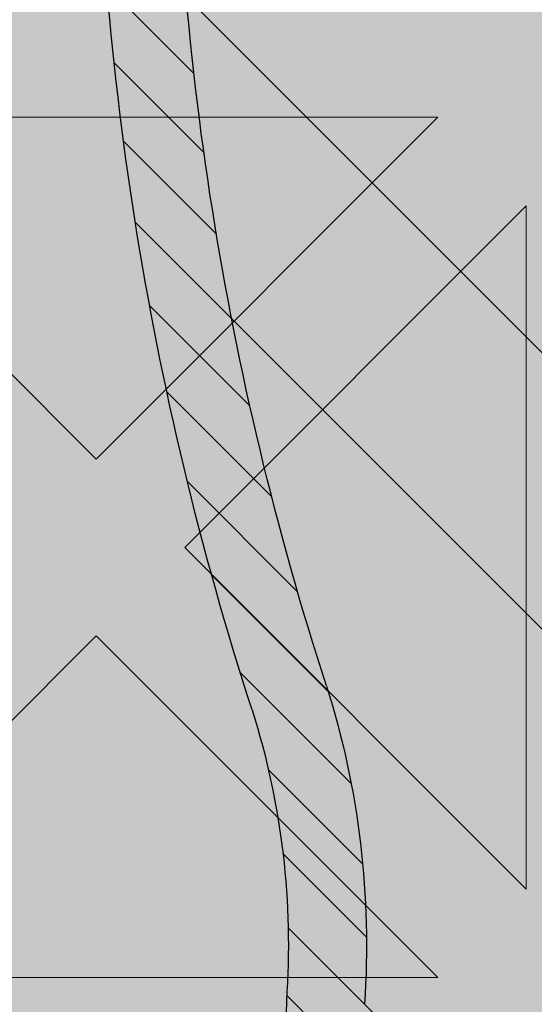
# Model space of a CAD drawing. Units: inches. Extents: x 844 to 2234, y 346 to 1084.
# Tile 70 of 93: x 2000.116 to 2001.166, y 694.327 to 696.335. Entities that reach past the tile are written whole.
import ezdxf

# ---------------------------------------------------------------- set-up
doc = ezdxf.new("R2010")
doc.units = ezdxf.units.IN
doc.header["$MEASUREMENT"] = 0
for name, color, linetype, lineweight in [('A-ANNO-DIMS', 2, 'Continuous', 18), ('furniture', 8, 'Continuous', 18), ('RA-AP-01$0$INT', 35, 'Continuous', 5)]:
    doc.layers.add(name, color=color, linetype=linetype, lineweight=lineweight)
doc.layers.add('RA-AP-01$0$FURN', color=3, linetype='Continuous')
doc.layers.add('RA-AP-01$0$WOOD', color=64, linetype='Continuous')
doc.styles.get("Standard").update_dxf_attribs({"font": 'arial.ttf'})
doc.dimstyles.get("Standard").update_dxf_attribs({"dimtxt": 6, "dimasz": 3, "dimexe": 0.18, "dimexo": 0.0625, "dimgap": 0.09, "dimtad": 0, "dimtih": 1, "dimtoh": 1, "dimdec": 1, "dimzin": 0, "dimdsep": 46, "dimlunit": 3, "dimtxsty": 'Standard', "dimblk": 'ARCHTICK', "dimcen": 0.09, "dimadec": 0, "dimazin": 0, "dimtfac": 1, "dimtdec": 1, "dimtofl": 0, "dimtmove": 0, "dimatfit": 3, "dimfxl": 1, "dimtolj": 1, "dimtzin": 0, "dimarcsym": 0})

# ---------------------------------------------------------------- blocks, each defined once
blk = doc.blocks.new('A$C18D01794')
at = {"layer": 'RA-AP-01$0$INT'}
h = blk.add_hatch(color=256, dxfattribs=at)
h.paths.add_polyline_path([(4.585917135068448, -6.356712009588273), (4.614201406330596, -6.356712009589021), (4.668846067270487, -6.411356670531338), (4.723490728212344, -6.356712009591912), (4.771774999457151, -6.35671200959319), (4.826419660396886, -6.411356670535356), (4.862780050090322, -6.374996280843536), (4.844495778842715, -6.356712009595112), (4.862780050090411, -6.356712009595595), (4.905206456960182, -6.399138416468211), (4.947632863832445, -6.356712009597838), (4.965917135079675, -6.356712009598322), (4.947632863831759, -6.374996280845421), (4.983993253523576, -6.411356670538857), (5.038637914464627, -6.356712009600247), (5.08692218571208, -6.356712009601523), (5.141566846649976, -6.411356670541852), (5.196211507589851, -6.356712009604411), (5.224495778822615, -6.356712009605161), (4.905206456953975, -6.676001331473793)])
h.paths.add_polyline_path([(4.895206456956031, -6.637717060225675), (4.895206456958921, -6.528427738347902), (4.840561796018589, -6.583072399285802)], flags=16)
h.paths.add_polyline_path([(4.915206456955638, -6.637717060226121), (4.969851117895509, -6.583072399288678), (4.915206456957609, -6.528427738348344)], flags=16)
h.paths.add_polyline_path([(4.826419660395175, -6.568930263661755), (4.881064321335613, -6.514285602723745), (4.771774999456703, -6.514285602720857)], flags=16)
h.paths.add_polyline_path([(4.983993253519558, -6.568930263665262), (5.038637914460456, -6.514285602726792), (4.929348592581548, -6.514285602724816)], flags=16)
h.paths.add_polyline_path([(4.881064321336025, -6.494285602723742), (4.826419660397532, -6.439640941782821), (4.771774999457062, -6.494285602720859)], flags=16)
h.paths.add_polyline_path([(4.929348592582019, -6.494285602724817), (5.038637914460982, -6.494285602726792), (4.983993253522945, -6.439640941786327)], flags=16)
h.paths.add_polyline_path([(4.895206456960191, -6.480143467100443), (4.895206456962115, -6.407422687715913), (4.876922185715016, -6.389138416467584), (4.840561796021581, -6.425498806159401)], flags=16)
h.paths.add_polyline_path([(4.915206456958487, -6.480143467100889), (4.969851117899527, -6.425498806162279), (4.933490728206909, -6.389138416468043), (4.9152064569598, -6.40742268771434)], flags=16)
h.paths.add_polyline_path([(4.757632863832376, -6.480143467096812), (4.812277524772842, -6.425498806158772), (4.757632863834348, -6.370854145217844)], flags=16)
h.paths.add_polyline_path([(4.737632863832376, -6.480143467096286), (4.737632863834348, -6.370854145217375), (4.682988202893906, -6.425498806155385)], flags=16)
h.paths.add_polyline_path([(5.05278005008503, -6.480143467103376), (5.052780050087917, -6.370854145224413), (4.998135389146995, -6.425498806162908)], flags=16)
h.paths.add_polyline_path([(5.072780050085024, -6.480143467103744), (5.127424711025931, -6.42549880616527), (5.072780050087916, -6.370854145224832)], flags=16)
h.paths.add_polyline_path([(4.935917135072783, -6.706712009592292), (5.255206456948811, -6.387422687716309), (5.255206456948932, -6.415706958964177), (5.200561796010279, -6.470351619902839), (5.255206456949403, -6.524996280841948), (5.25520645694961, -6.5732805520894), (5.200561796009787, -6.627925213029239), (5.236922185702417, -6.664285602721864), (5.255206456949919, -6.646001331474357), (5.255206456949998, -6.664285602721898), (5.212780050078687, -6.706712009592262), (5.25520645695036, -6.749138416463932), (5.255206456950438, -6.767422687711313), (5.236922185702424, -6.749138416463297), (5.200561796009796, -6.785498806155928), (5.255206456950753, -6.840143467096874), (5.25520645695096, -6.888427738341682), (5.200561796010322, -6.943072399282328), (5.255206456951428, -6.997717060223427), (5.255206456951547, -7.026001331471006)])
h.paths.add_polyline_path([(5.042988202883395, -6.785498806155427), (5.097632863823085, -6.840143467095101), (5.097632863822622, -6.730854145216193)], flags=16)
h.paths.add_polyline_path([(5.028846067259663, -6.771356670531693), (5.083490728198774, -6.716712009592573), (4.974201406321001, -6.716712009593042)], flags=16)
h.paths.add_polyline_path([(5.117632863823087, -6.840143467095186), (5.172277524762331, -6.785498806155926), (5.11763286382262, -6.730854145216225)], flags=16)
h.paths.add_polyline_path([(5.08349072819877, -6.696712009593886), (5.028846067259652, -6.642067348654775), (4.974201406320998, -6.696712009593438)], flags=16)
h.paths.add_polyline_path([(5.131774999446817, -6.854285602718917), (5.186419660386065, -6.799640941779662), (5.241064321325782, -6.854285602719365)], flags=17)
h.paths.add_polyline_path([(5.131774999446228, -6.716712009592374), (5.186419660386065, -6.771356670532194), (5.222780050079488, -6.734996280838764), (5.204495778832781, -6.716712009592063)], flags=16)
h.paths.add_polyline_path([(5.097632863822613, -6.682569873970264), (5.097632863823061, -6.573280552091354), (5.042988202883383, -6.627925213031044)], flags=16)
h.paths.add_polyline_path([(5.131774999446899, -6.874285602718915), (5.241064321325809, -6.874285602719364), (5.186419660386591, -6.928930263658598)], flags=17)
h.paths.add_polyline_path([(5.131774999446226, -6.696712009594078), (5.204495778830767, -6.696712009594374), (5.22278005007868, -6.67842773834687), (5.186419660386049, -6.642067348654249)], flags=16)
h.paths.add_polyline_path([(5.11763286382262, -6.682569873970225), (5.17227752476232, -6.627925213030515), (5.117632863823064, -6.573280552091267)], flags=16)
h.paths.add_polyline_path([(5.186419660386069, -6.613783077405491), (5.241064321325754, -6.559138416465795), (5.131774999446791, -6.559138416466263)], flags=16)
h.paths.add_polyline_path([(5.131774999446872, -6.539138416466263), (5.24106432132578, -6.539138416465794), (5.186419660386554, -6.484493755526573)], flags=16)
h.paths.add_polyline_path([(5.255206456951811, -7.08742268770861), (5.255206456951895, -7.106712009588038), (4.555206456956052, -7.106712009588038), (4.555206456956136, -7.087422687708617), (4.905206456953973, -6.737422687710788)])
h.paths.add_polyline_path([(4.983993253513404, -6.8444937555241), (4.92934859257295, -6.899138416462108), (5.03863791445186, -6.899138416465014)], flags=16)
h.paths.add_polyline_path([(4.969851117889988, -6.83035161990006), (4.915206456952556, -6.775706958960171), (4.915206456949648, -6.884996280837944)], flags=16)
h.paths.add_polyline_path([(4.929348592572535, -6.919138416462105), (4.983993253511019, -6.973783077403037), (5.038637914451496, -6.919138416465012)], flags=16)
h.paths.add_polyline_path([(5.052780050074912, -6.93328055208906), (4.998135389134438, -6.987925213027088), (5.052780050072919, -7.042569873968025)], flags=16)
h.paths.add_polyline_path([(5.07278005007491, -6.933280552089588), (5.072780050072918, -7.042569873968497), (5.127424711013374, -6.987925213030498)], flags=16)
h.paths.add_polyline_path([(4.89520645695295, -6.775706958959721), (4.840561796013067, -6.830351619897157), (4.895206456950961, -6.884996280837494)], flags=16)
h.paths.add_polyline_path([(4.915206456948365, -6.933280552085403), (4.915206456946434, -7.006001331471951), (4.933490728192729, -7.024285602719066), (4.969851117886972, -6.987925213026453)], flags=16)
h.paths.add_polyline_path([(4.881064321327021, -6.899138416461022), (4.82641966038902, -6.84449375552057), (4.771774999448108, -6.899138416459029)], flags=16)
h.paths.add_polyline_path([(4.895206456950073, -6.933280552084951), (4.840561796009022, -6.987925213023558), (4.876922185700835, -7.024285602716997), (4.895206456948749, -7.006001331469487)], flags=16)
h.paths.add_polyline_path([(4.983993253510392, -7.0020673486505), (4.947632863816944, -7.038427738342319), (4.965917135064043, -7.05671200959023), (5.038637914448995, -7.056712009591555)], flags=16)
h.paths.add_polyline_path([(4.881064321326543, -6.91913841646102), (4.771774999447578, -6.919138416459031), (4.826419660385607, -6.973783077399508)], flags=16)
h.paths.add_polyline_path([(4.905206456946447, -7.014285602717636), (4.862780050074785, -7.056712009588352), (4.947632863816685, -7.056712009589775)], flags=16)
h.paths.add_polyline_path([(5.14156684663679, -7.002067348654549), (5.086922185696452, -7.056712009592438), (5.196211507574223, -7.056712009594425)], flags=16)
h.paths.add_polyline_path([(4.8264196603837, -7.002067348646972), (4.771774999442643, -7.056712009585575), (4.8444957788276, -7.056712009587508), (4.862780050075511, -7.038427738340416)], flags=16)
h.paths.add_polyline_path([(4.812277524760289, -6.98792521302292), (4.757632863822258, -6.933280552082447), (4.757632863819352, -7.042569873961408)], flags=16)
h.paths.add_polyline_path([(4.73763286382226, -6.933280552082079), (4.682988202881349, -6.987925213020536), (4.737632863819352, -7.04256987396099)], flags=16)
h.paths.add_polyline_path([(4.723490728195188, -7.056712009584289), (4.668846067257299, -7.002067348643949), (4.614201406317417, -7.056712009581383)], flags=16)
h.paths.add_polyline_path([(4.597632863829262, -6.706712009592262), (4.555206456957951, -6.664285602721896), (4.555206456958029, -6.646001331474357), (4.573490728205535, -6.664285602721864), (4.609851117898167, -6.627925213029238), (4.555206456958338, -6.573280552089402), (4.555206456958546, -6.524996280841952), (4.60985111789767, -6.470351619902839), (4.555206456959015, -6.415706958964177), (4.555206456959138, -6.387422687716309), (4.874495778835167, -6.70671200959229), (4.5552064569564, -7.026001331471015), (4.555206456956523, -6.997717060223433), (4.609851117897629, -6.94307239928233), (4.555206456956988, -6.888427738341681), (4.555206456957198, -6.840143467096881), (4.609851117898153, -6.78549880615593), (4.573490728205528, -6.749138416463297), (4.555206456957507, -6.76742268771132), (4.555206456957585, -6.749138416463933)])
h.paths.add_polyline_path([(4.712780050085332, -6.730854145216195), (4.712780050084863, -6.840143467095105), (4.767424711024555, -6.785498806155427)], flags=16)
h.paths.add_polyline_path([(4.726922185709173, -6.716712009592573), (4.781566846648288, -6.771356670531693), (4.836211507586949, -6.716712009593043)], flags=16)
h.paths.add_polyline_path([(4.692780050085327, -6.730854145216225), (4.638135389145619, -6.785498806155928), (4.692780050084865, -6.840143467095185)], flags=16)
h.paths.add_polyline_path([(4.726922185709182, -6.696712009593886), (4.836211507586949, -6.696712009593436), (4.7815668466483, -6.642067348654773)], flags=16)
h.paths.add_polyline_path([(4.678637914461726, -6.71671200959237), (4.605917135075169, -6.716712009592063), (4.587632863828464, -6.734996280838766), (4.623993253521887, -6.771356670532195)], flags=16)
h.paths.add_polyline_path([(4.712780050085336, -6.68256987397026), (4.767424711024568, -6.627925213031042), (4.71278005008489, -6.573280552091352)], flags=16)
h.paths.add_polyline_path([(4.678637914461726, -6.696712009594076), (4.623993253521899, -6.642067348654247), (4.587632863829271, -6.67842773834687), (4.605917135077185, -6.696712009594376)], flags=16)
h.paths.add_polyline_path([(4.692780050085336, -6.682569873970228), (4.692780050084889, -6.573280552091267), (4.638135389145632, -6.627925213030515)], flags=16)
h.paths.add_polyline_path([(4.623993253521885, -6.799640941779662), (4.678637914461131, -6.854285602718915), (4.56934859258217, -6.854285602719365)], flags=17)
h.paths.add_polyline_path([(4.623993253521901, -6.613783077405509), (4.678637914461158, -6.559138416466263), (4.569348592582195, -6.559138416465795)], flags=16)
h.paths.add_polyline_path([(4.678637914461051, -6.874285602718915), (4.623993253521361, -6.928930263658598), (4.569348592582143, -6.874285602719364)], flags=17)
h.paths.add_polyline_path([(4.678637914461076, -6.539138416466263), (4.623993253521399, -6.484493755526573), (4.569348592582167, -6.539138416465796)], flags=16)
h = blk.add_hatch(color=256, dxfattribs=at)
h.paths.add_polyline_path([(5.028846067259997, -6.642067348655121), (4.974201406321342, -6.696712009593783), (5.083490728199115, -6.69671200959423)])
h.paths.add_polyline_path([(4.974201406321344, -6.716712009593388), (5.028846067260004, -6.771356670532039), (5.083490728199117, -6.716712009592919)])
h.paths.add_polyline_path([(5.042988202883738, -6.785498806155768), (5.097632863823428, -6.840143467095449), (5.097632863822963, -6.73085414521654)])
h.paths.add_polyline_path([(5.117632863822961, -6.730854145216568), (5.117632863823428, -6.840143467095531), (5.172277524762674, -6.785498806156272)])
h.paths.add_polyline_path([(5.131774999446572, -6.716712009592718), (5.186419660386406, -6.77135667053254), (5.222780050079831, -6.734996280839116), (5.204495778833122, -6.716712009592409)])
h.paths.add_polyline_path([(5.236922185702764, -6.749138416463644), (5.200561796010139, -6.785498806156274), (5.255206456949971, -6.840143467096101), (5.255206456950271, -6.76742268771115)])
h.paths.add_polyline_path([(5.186419660386412, -6.799640941780006), (5.131774999447164, -6.854285602719262), (5.241064321326123, -6.854285602719711)])
h.paths.add_polyline_path([(5.131774999447238, -6.874285602719261), (5.186419660386934, -6.928930263658944), (5.241064321326153, -6.874285602719709)])
h.paths.add_polyline_path([(5.200561796010663, -6.943072399282675), (5.255206456949324, -6.997717060221329), (5.255206456949777, -6.888427738343558)])
h.paths.add_polyline_path([(5.21278005007903, -6.706712009592607), (5.255206456950223, -6.749138416463798), (5.255206456950696, -6.664285602721891)])
h.paths.add_polyline_path([(5.13177499944657, -6.696712009594424), (5.204495778831106, -6.696712009594723), (5.222780050079024, -6.678427738347219), (5.186419660386397, -6.642067348654592)])
h.paths.add_polyline_path([(5.117632863823405, -6.573280552091611), (5.117632863822955, -6.682569873970578), (5.172277524762665, -6.627925213030859)])
h.paths.add_polyline_path([(5.042988202883727, -6.627925213031387), (5.097632863822957, -6.682569873970603), (5.097632863823407, -6.573280552091697)])
h.paths.add_polyline_path([(5.131774999447135, -6.559138416466609), (5.186419660386394, -6.613783077405857), (5.241064321326097, -6.559138416466144)])
h.paths.add_polyline_path([(5.200561796010128, -6.627925213029584), (5.236922185702758, -6.664285602722211), (5.255206456950264, -6.646001331474705), (5.255206456949948, -6.573280552089752)])
h.paths.add_polyline_path([(5.186419660386895, -6.484493755526919), (5.131774999447213, -6.539138416466609), (5.241064321326127, -6.539138416466142)])
h.paths.add_polyline_path([(5.200561796010624, -6.470351619903183), (5.255206456949745, -6.524996280842298), (5.255206456949276, -6.415706958964523)])
for p, q in [((5.131774999446792, -6.559138416466263), (5.241064321325755, -6.559138416465795)), ((5.131774999446792, -6.559138416466263), (5.186419660386049, -6.613783077405509)), ((5.241064321325755, -6.559138416465795), (5.186419660386049, -6.613783077405509)), ((5.117632863823062, -6.573280552091267), (5.172277524762319, -6.627925213030515)), ((5.117632863823062, -6.573280552091267), (5.117632863822614, -6.68256987397023)), ((5.117632863822614, -6.68256987397023), (5.172277524762319, -6.627925213030515)), ((5.131774999446228, -6.696712009594078), (5.186419660386053, -6.642067348654247)), ((5.186419660386051, -6.642067348654247), (5.222780050078681, -6.67842773834687)), ((5.204495778831179, -6.696712009594376), (5.131774999446228, -6.696712009594078))]:
    blk.add_line(p, q, dxfattribs=at)
blk = doc.blocks.new('A$C32926AE1')
at = {"layer": 'RA-AP-01$0$WOOD'}
h = blk.add_hatch(color=256, dxfattribs=at)
h.dxf.hatch_style = 1
h.paths.add_polyline_path([(5.157430609644524, 4.573483066760929, -0.1009492694046607), (5.155401577623758, 4.593365984175333, -0.1842662638101597), (5.172249623284174, 4.638795604568598, 0.2056608120311276), (5.179560981299304, 4.661316324430096, 0.3614336704623542), (5.134352340494423, 4.706524965234944, 0.2056608120311297), (5.111831620632933, 4.699213607219793, -0.1842662638101113), (5.066402000239693, 4.682365561559342, -0.1055311479399994), (5.045656153913092, 4.68467289944697, 0.1567636581983829), (4.763886414745334, 4.684672899446966, -0.1055311479399895), (4.743140568418733, 4.68236556155934, -0.1842662638100833), (4.6977109480255, 4.69921360721979, 0.2056608120302612), (4.675190228164109, 4.706524965234949, 0.3614336704708441), (4.629981587358889, 4.66131632442871, 0.2056608120245944), (4.637292945374126, 4.638795604567974, -0.1842662638101024), (4.654140991034615, 4.59336598417475, -0.1009492694055169), (4.652111959013835, 4.573483066760181, 0.021410119221476), (4.629748025606143, 4.156712009541676, 0.0214101192214795), (4.652111959013809, 3.739940952323101, -0.1009492694059586), (4.654140991034615, 3.720058034908448, -0.1842662638100975), (4.637292945374126, 3.674628414515226, 0.2056608120245705), (4.629981587358889, 3.652107694654492, 0.3614336704708879), (4.675190228164113, 3.606899053848249, 0.2056608120302384), (4.697710948025501, 3.614210411863408, -0.1842662638100995), (4.743140568418738, 3.63105845752386, -0.1055311479402541), (4.763886414745388, 3.628751119636215, 0.1567636581983776), (5.045656153913137, 3.628751119636244, -0.1055311479397538), (5.066402000239692, 3.631058457523857, -0.1842662638101067), (5.111831620632931, 3.614210411863407, 0.2056608120310924), (5.134352340494417, 3.606899053848256, 0.3614336704624001), (5.179560981299307, 3.652107694653103, 0.2056608120311314), (5.172249623284175, 3.6746284145146, -0.1842662638101402), (5.155401577623758, 3.72005803490786, -0.1009492694051366), (5.15743060964455, 3.739940952322354, 0.0214101192215073), (5.179794543052287, 4.156712009541468, 0.0214101192215252)])
h.paths.add_polyline_path([(4.639748609479751, 4.156712009541513, 0.0213537860821624), (4.661970494867118, 3.741887061152232, -0.094075836301374), (4.664143710413708, 3.7196126951003, -0.1824818158568985), (4.644813765429836, 3.668037719127816, 0.2056608120245319), (4.639939526753007, 3.653023905887301, 0.3614336704710246), (4.676106439397173, 3.616856993242342, 0.2056608120302234), (4.691120252638095, 3.621731231919122, -0.1824818158602558), (4.742695228611606, 3.641061176902986, -0.1029891339458722), (4.766991894714349, 3.638256818950944, 0.156709409989566), (5.042550673941472, 3.638256818950105, -0.102989133958497), (5.066847340047078, 3.641061176902949, -0.1824818158594995), (5.118422316020358, 3.621731231919103, 0.2056608120311416), (5.133436129261316, 3.616856993242346, 0.3614336704621468), (5.169603041905217, 3.653023905886178, 0.2056608120310986), (5.164728803228477, 3.668037719127177, -0.1824818158565612), (5.145398858244737, 3.719612695099578, -0.0940758363009313), (5.147572073791232, 3.741887061151398, 0.0213537860822023), (5.169793959178681, 4.156712009541451, 0.0213537860822226), (5.147572073791203, 4.571536957931898, -0.0940758363005034), (5.145398858244737, 4.59381132398362, -0.1824818158565587), (5.164728803228476, 4.645386299956021, 0.2056608120311045), (5.169603041905216, 4.66040011319702, 0.3614336704621845), (5.133436129261313, 4.696567025840856, 0.2056608120310773), (5.118422316020359, 4.691692787164098, -0.182481815859508), (5.066847340047078, 4.67236284218025, -0.1029891339584606), (5.04255067394148, 4.675167200133092, 0.156709409989566), (4.766991894714357, 4.675167200132257, -0.1029891339458842), (4.742695228611611, 4.672362842180213, -0.1824818158602725), (4.691120252638095, 4.691692787164077, 0.2056608120302152), (4.676106439397174, 4.696567025840858, 0.3614336704710363), (4.639939526753005, 4.660400113195899, 0.2056608120245495), (4.644813765429837, 4.645386299955384, -0.1824818158568934), (4.664143710413708, 4.593811323982902, -0.0940758363009187), (4.661970494867149, 4.571536957931074, 0.021353786082177)], flags=16)
h.paths.add_polyline_path([(5.129794543052235, 4.432167055276933, -0.0141661062790638), (5.130152669293814, 4.156927903047693, -0.0141661062790647), (5.129794543052234, 3.881688750818433, -0.0785247771143638), (5.10979738006795, 3.755143611847103, 0.0945969212073497), (5.105408519571111, 3.717898134952927, 0.1043170707844957), (5.116074640131521, 3.670385395016088, 0.1043170707864965), (5.068561900193738, 3.681051515576561, 0.09459692119553), (5.031316423304057, 3.676662655080835, -0.1580239521427272), (4.778226145355827, 3.676662655080367, 0.0945969211986668), (4.740980668464973, 3.681051515576592, 0.1043170707882822), (4.693467928526415, 3.670385395015844, 0.1043170707867916), (4.704134049087309, 3.717898134953662, 0.0945969211972894), (4.69974518859162, 3.755143611844042, -0.0785247771163196), (4.679748025606343, 3.881688750818406, -0.0141661062790663), (4.679389899364763, 4.156927903047693, -0.0141661062790672), (4.679748025606343, 4.432167055276998, -0.0785247771163064), (4.699745188591625, 4.55871219425134, 0.094596921197333), (4.704134049087308, 4.595957671141738, 0.1043170707867205), (4.693467928526416, 4.643470411079523, 0.1043170707882628), (4.740980668464965, 4.632804290518776, 0.0945969211988114), (4.778226145355874, 4.637193151015016, -0.158023952142669), (5.031316423304015, 4.637193151014546, 0.0945969211956361), (5.068561900193736, 4.632804290518806, 0.1043170707864979), (5.11607464013152, 4.643470411079278, 0.1043170707844617), (5.105408519571112, 4.595957671142455, 0.0945969212074597), (5.109797380067959, 4.558712194248236, -0.0785247771143467)], flags=0)
h.paths.add_polyline_path([(5.119794532311105, 4.432259799204851, -0.0142000800617244), (5.120156169157484, 4.156927903047701, -0.0142000800617277), (5.119794532311105, 3.881596006890482, -0.0784894509520253), (5.100273383573699, 3.758192358677797, 0.0940138827242913), (5.095413455884425, 3.717477693979438, 0.0606271852308753), (5.099615656341024, 3.686844378806616, 0.0606271852322524), (5.068982341167493, 3.691046579263239, 0.0940138827010453), (5.028267676478798, 3.686186651576848, -0.1580706864508061), (4.781274892180912, 3.686186651576435, 0.0940138827026903), (4.740560227491556, 3.691046579263279, 0.0606271852339895), (4.709926912317155, 3.686844378806508, 0.0606271852329405), (4.714129112773991, 3.717477693980356, 0.094013882701304), (4.709269185087677, 3.758192358669163, -0.0784894509577193), (4.689748036347473, 3.881596006890469, -0.014200080061729), (4.689386399501094, 4.156927903047709, -0.0142000800617217), (4.689748036347473, 4.432259799204808, -0.078489450957724), (4.709269185087651, 4.555663447426125, 0.0940138827014585), (4.714129112773992, 4.596378112114996, 0.0606271852329731), (4.709926912317154, 4.62701142728886, 0.0606271852340196), (4.74056022749157, 4.622809226832087, 0.0940138827024997), (4.781274892180847, 4.627669154518912, -0.1580706864508359), (5.028267676478777, 4.627669154518526, 0.0940138827010946), (5.068982341167492, 4.622809226832129, 0.060627185232254), (5.099615656341024, 4.627011427288751, 0.0606271852308727), (5.095413455884425, 4.59637811211593, 0.0940138827241088), (5.100273383573675, 4.555663447417647, -0.0784894509520978)], flags=0)
h.paths.add_polyline_path([(5.06978912287499, 4.430218106756144, -0.014241683694547), (5.070173729147532, 4.156927903047672, -0.0142416836945458), (5.06978912287499, 3.883637699339223, -0.0800609523125196), (5.052662118612511, 3.773463122773442, 0.0526421978001116), (5.04590916754064, 3.740550867606997, 0.0526421977992423), (5.012996912374707, 3.73379791653534, -0.1583028414718258), (4.796545656286308, 3.73379791653451, 0.0526421978034211), (4.763633401117837, 3.740550867607021, 0.0526421978018622), (4.756880450045755, 3.773463122774558, -0.0800609523117106), (4.739753445783639, 3.883637699339268, -0.0142416836945435), (4.739368839511098, 4.156927903047671, -0.0142416836945477), (4.739753445783639, 4.430218106756155, -0.0800609523116345), (4.75688045004574, 4.540392683320762, 0.052642197801941), (4.763633401117837, 4.573304938488346, 0.0526421978035071), (4.796545656286361, 4.580057889560873, -0.1583028414717561), (5.012996912374669, 4.580057889560039, 0.0526421977993048), (5.04590916754064, 4.57330493848837, 0.0526421978002057), (5.052662118612529, 4.540392683321868, -0.080060952312477)], flags=0)
h.paths.add_polyline_path([(5.049789715110557, 4.43038092723357, -0.0143097550741839), (5.05018085590259, 4.156927903047715, -0.0143097550741854), (5.049789715110558, 3.883474878861827, -0.0800685599149176), (5.03362098255317, 3.779581877367999, 0.0306258898956367), (5.028241146483733, 3.758218888663947, 0.0306258898977031), (5.006878157778253, 3.75283905259408, -0.1583983521624096), (4.802664410878162, 3.752839052594731, 0.0306258898946014), (4.781301422174808, 3.758218888663924, 0.0306258898967912), (4.775921586105202, 3.779581877368794, -0.080068559914251), (4.759752853548071, 3.883474878861786, -0.0143097550741854), (4.759361712756037, 4.156927903047671, -0.0143097550741854), (4.759752853548071, 4.430380927233557, -0.0800685599142479), (4.775921586105193, 4.534273928726546, 0.0306258898968306), (4.781301422174808, 4.555636917431444, 0.0306258898945754), (4.802664410878143, 4.561016753500631, -0.1583983521624168), (5.006878157778244, 4.561016753501291, 0.0306258898977177), (5.028241146483733, 4.555636917431421, 0.0306258898958182), (5.03362098255321, 4.534273928727244, -0.080068559914796)], flags=0)
h.paths.add_polyline_path([(4.999766070382627, 4.428171244713864, -0.0143443147609634), (5.000198441819402, 4.156927903047689, -0.0143443147609612), (4.999766070382627, 3.885684561381556, -0.0784641635803329), (4.987356730658798, 3.799103304488872, -0.1506053783831347), (4.822185837999821, 3.79910330448882, -0.0784641635803318), (4.809776498276007, 3.885684561381509, -0.014344314760963), (4.809344126839227, 4.156927903047677, -0.0143443147609645), (4.809776498276007, 4.428171244713873, -0.0784641635803192), (4.822185837999822, 4.514752501606549, -0.1506053783831338), (4.987356730658798, 4.514752501606494, -0.078464163580285)], flags=0)
h.paths.add_polyline_path([(4.979755254238824, 4.42764379880488, -0.0143772539198268), (4.980205517789977, 4.156927903047693, -0.0143772539198275), (4.979755254238824, 3.886212007290489, -0.0689242507424422), (4.971183264704897, 3.815276770442801, -0.1296645318904179), (4.838359303953726, 3.815276770442746, -0.0689242507424186), (4.829787314419809, 3.886212007290419, -0.0143772539198292), (4.829337050868653, 4.156927903047653, -0.0143772539198325), (4.829787314419809, 4.427643798804946, -0.0689242507424211), (4.838359303953725, 4.498579035652621, -0.1296645318904187), (4.971183264704897, 4.498579035652565, -0.0689242507424401)], flags=0)
h = blk.add_hatch(color=256, dxfattribs=at)
h.dxf.hatch_style = 1
h.paths.add_polyline_path([(5.145398858244737, 4.59381132398362, -0.1824818158565616), (5.164728803228476, 4.645386299956021, 0.2056608120311045), (5.169603041905216, 4.66040011319702, 0.3614336704621845), (5.133436129261313, 4.696567025840856, 0.2056608120310773), (5.118422316020359, 4.691692787164098, -0.182481815859508), (5.066847340047078, 4.67236284218025, -0.1029891339584606), (5.04255067394148, 4.675167200133092, 0.156709409989566), (4.766991894714357, 4.675167200132257, -0.1029891339458842), (4.742695228611611, 4.672362842180213, -0.1824818158602725), (4.691120252638095, 4.691692787164077, 0.2056608120302152), (4.676106439397174, 4.696567025840858, 0.3614336704710363), (4.639939526753005, 4.660400113195899, 0.2056608120245495), (4.644813765429837, 4.645386299955384, -0.1824818158568934), (4.664143710413708, 4.593811323982902, -0.0940758363009187), (4.661970494867149, 4.571536957931074, 0.0213537860821772), (4.639748609479751, 4.156712009541507, 0.0213537860821625), (4.661970494867119, 3.741887061152226, -0.0940758363013071), (4.664143710413708, 3.719612695100309, -0.1824818158569294), (4.644813765429836, 3.668037719127816, 0.2056608120245319), (4.639939526753007, 3.653023905887301, 0.3614336704710246), (4.676106439397173, 3.616856993242342, 0.2056608120302234), (4.691120252638095, 3.621731231919122, -0.1824818158602558), (4.742695228611606, 3.641061176902986, -0.1029891339458722), (4.766991894714349, 3.638256818950944, 0.156709409989566), (5.042550673941472, 3.638256818950105, -0.102989133958497), (5.066847340047078, 3.641061176902949, -0.1824818158594995), (5.118422316020358, 3.621731231919103, 0.2056608120311416), (5.133436129261316, 3.616856993242346, 0.3614336704621468), (5.169603041905217, 3.653023905886178, 0.2056608120310986), (5.164728803228477, 3.668037719127177, -0.1824818158565612), (5.145398858244737, 3.719612695099578, -0.0940758363009313), (5.147572073791232, 3.741887061151398, 0.0213537860822023), (5.169793959178681, 4.156712009541451, 0.0213537860822226), (5.147572073791203, 4.571536957931898, -0.0940758363004996)])
h.paths.add_polyline_path([(5.109797380067958, 4.55871219424824, -0.0785247771143472), (5.129794543052234, 4.432167055276936, -0.0141661062790644), (5.130152669293814, 4.156927903047685, -0.014166106279066), (5.129794543052234, 3.881688750818401, -0.0785247771143517), (5.109797380067946, 3.755143611847092, 0.0945969212073132), (5.105408519571111, 3.717898134952929, 0.1043170707844995), (5.116074640131521, 3.670385395016088, 0.1043170707864965), (5.068561900193738, 3.681051515576561, 0.09459692119553), (5.031316423304057, 3.676662655080835, -0.1580239521427272), (4.778226145355827, 3.676662655080367, 0.0945969211986668), (4.740980668464973, 3.681051515576592, 0.1043170707882822), (4.693467928526415, 3.670385395015844, 0.1043170707867916), (4.704134049087309, 3.717898134953662, 0.0945969211972894), (4.69974518859162, 3.755143611844042, -0.0785247771163196), (4.679748025606343, 3.881688750818406, -0.0141661062790663), (4.679389899364763, 4.156927903047693, -0.0141661062790672), (4.679748025606343, 4.432167055276998, -0.0785247771163064), (4.699745188591625, 4.55871219425134, 0.094596921197333), (4.704134049087308, 4.595957671141738, 0.1043170707867205), (4.693467928526416, 4.643470411079523, 0.1043170707882628), (4.740980668464965, 4.632804290518776, 0.0945969211988114), (4.778226145355874, 4.637193151015016, -0.158023952142669), (5.031316423304015, 4.637193151014546, 0.0945969211956361), (5.068561900193736, 4.632804290518806, 0.1043170707864979), (5.11607464013152, 4.643470411079278, 0.1043170707844617), (5.105408519571112, 4.595957671142455, 0.0945969212074504)], flags=16)
h.paths.add_polyline_path([(5.100273383573655, 4.55566344741771, -0.0784894509521388), (5.119794532311105, 4.432259799204852, -0.0142000800617252), (5.120156169157484, 4.156927903047686, -0.014200080061726), (5.119794532311105, 3.881596006890502, -0.0784894509520446), (5.100273383573696, 3.758192358677786, 0.0940138827242721), (5.095413455884425, 3.717477693979436, 0.0606271852308692), (5.099615656341024, 3.686844378806616, 0.0606271852322522), (5.068982341167493, 3.691046579263239, 0.0940138827010453), (5.028267676478798, 3.686186651576848, -0.1580706864508061), (4.781274892180912, 3.686186651576435, 0.0940138827026903), (4.740560227491556, 3.691046579263279, 0.0606271852339895), (4.709926912317155, 3.686844378806508, 0.0606271852329405), (4.714129112773991, 3.717477693980356, 0.094013882701304), (4.709269185087677, 3.758192358669163, -0.0784894509577193), (4.689748036347473, 3.881596006890469, -0.014200080061729), (4.689386399501094, 4.156927903047709, -0.0142000800617217), (4.689748036347473, 4.432259799204808, -0.078489450957724), (4.709269185087651, 4.555663447426125, 0.0940138827014585), (4.714129112773992, 4.596378112114996, 0.0606271852329731), (4.709926912317154, 4.62701142728886, 0.0606271852340196), (4.74056022749157, 4.622809226832087, 0.0940138827024997), (4.781274892180847, 4.627669154518912, -0.1580706864508359), (5.028267676478777, 4.627669154518526, 0.0940138827010946), (5.068982341167492, 4.622809226832129, 0.060627185232254), (5.099615656341024, 4.627011427288751, 0.0606271852308727), (5.095413455884425, 4.59637811211593, 0.094013882723957)], flags=0)
h.paths.add_polyline_path([(5.04590916754064, 4.57330493848837, 0.0526421978002057), (5.052662118612529, 4.540392683321868, -0.0800609523124783), (5.06978912287499, 4.430218106756142, -0.0142416836945469), (5.070173729147532, 4.156927903047672, -0.0142416836945458), (5.06978912287499, 3.883637699339223, -0.0800609523125196), (5.052662118612511, 3.773463122773442, 0.0526421978001116), (5.04590916754064, 3.740550867606997, 0.0526421977992423), (5.012996912374707, 3.73379791653534, -0.1583028414718258), (4.796545656286308, 3.73379791653451, 0.0526421978034211), (4.763633401117837, 3.740550867607021, 0.0526421978018622), (4.756880450045755, 3.773463122774558, -0.0800609523117106), (4.739753445783639, 3.883637699339268, -0.0142416836945435), (4.739368839511098, 4.156927903047671, -0.0142416836945477), (4.739753445783639, 4.430218106756155, -0.0800609523116345), (4.75688045004574, 4.540392683320762, 0.052642197801941), (4.763633401117837, 4.573304938488346, 0.0526421978035071), (4.796545656286361, 4.580057889560873, -0.1583028414717561), (5.012996912374669, 4.580057889560039, 0.0526421977993048)], flags=0)
h.paths.add_polyline_path([(5.028241146483733, 4.555636917431422, 0.0306258898956949), (5.033620982553182, 4.534273928727329, -0.0800685599148649), (5.049789715110557, 4.430380927233569, -0.0143097550741839), (5.05018085590259, 4.156927903047715, -0.0143097550741854), (5.049789715110558, 3.883474878861827, -0.0800685599149176), (5.03362098255317, 3.779581877367999, 0.0306258898956367), (5.028241146483733, 3.758218888663947, 0.0306258898977031), (5.006878157778253, 3.75283905259408, -0.1583983521624096), (4.802664410878162, 3.752839052594731, 0.0306258898946014), (4.781301422174808, 3.758218888663924, 0.0306258898967912), (4.775921586105202, 3.779581877368794, -0.080068559914251), (4.759752853548071, 3.883474878861786, -0.0143097550741854), (4.759361712756037, 4.156927903047671, -0.0143097550741854), (4.759752853548071, 4.430380927233557, -0.0800685599142479), (4.775921586105193, 4.534273928726546, 0.0306258898968306), (4.781301422174808, 4.555636917431444, 0.0306258898945754), (4.802664410878143, 4.561016753500631, -0.1583983521624168), (5.006878157778244, 4.561016753501291, 0.0306258898977174)], flags=0)
h.paths.add_polyline_path([(4.987356730658798, 4.514752501606494, -0.0784641635803018), (4.999766070382627, 4.428171244713845, -0.0143443147609637), (5.000198441819402, 4.156927903047665, -0.0143443147609622), (4.999766070382628, 3.885684561381514, -0.0784641635802952), (4.987356730658797, 3.799103304488872, -0.1506053783831338), (4.822185837999821, 3.799103304488819, -0.0784641635803342), (4.809776498276007, 3.885684561381512, -0.0143443147609628), (4.809344126839227, 4.156927903047676, -0.0143443147609646), (4.809776498276007, 4.428171244713873, -0.0784641635803192), (4.822185837999822, 4.514752501606549, -0.1506053783831338)], flags=0)
h.paths.add_polyline_path([(4.971183264704897, 4.498579035652566, -0.0689242507424384), (4.979755254238824, 4.427643798804883, -0.0143772539198276), (4.980205517789977, 4.15692790304768, -0.0143772539198258), (4.979755254238823, 3.88621200729051, -0.0689242507424628), (4.971183264704897, 3.815276770442801, -0.129664531890417), (4.838359303953726, 3.815276770442746, -0.0689242507424186), (4.829787314419809, 3.886212007290419, -0.0143772539198292), (4.829337050868653, 4.156927903047653, -0.0143772539198325), (4.829787314419809, 4.427643798804946, -0.0689242507424211), (4.838359303953725, 4.498579035652621, -0.1296645318904187)], flags=0)
h = blk.add_hatch(dxfattribs=at)
h.set_pattern_fill('ANSI31', color=256, scale=0.05, style=0)
h.set_pattern_definition([(45, (0, 0), (-0.0044194173824159, 0.0044194173824159), [])])
h.paths.add_polyline_path([(5.130152669293814, 4.156927903047704, 0.0141661062790657), (5.129794543052234, 4.432167055276982, 0.0777827904001433), (5.110168979996553, 4.557559993161921, -0.0976515123401879), (5.105408519571111, 4.595957671142454, -0.1043170707844687), (5.116074640131522, 4.64347041107928), (5.099615656341024, 4.627011427288751, 0.0606271852308727), (5.095413455884425, 4.59637811211593, 0.0940138827241088), (5.100273383573675, 4.555663447417647, -0.0784894509520972), (5.119794532311105, 4.432259799204852, -0.0142000800617252), (5.120156169157484, 4.156927903047686, -0.014200080061726), (5.119794532311105, 3.881596006890502, -0.0784894509520446), (5.100273383573696, 3.758192358677786, 0.0940138827242721), (5.095413455884425, 3.717477693979436, 0.0606271852308692), (5.099615656341024, 3.686844378806616), (5.116074640131519, 3.67038539501609, -0.1043170707844594), (5.105408519571112, 3.717898134952912, -0.0976515123401594), (5.11016897999655, 3.756295812933435, 0.0777827904001654), (5.129794543052234, 3.881688750818409, 0.0141661062790665)])
h.paths.add_polyline_path([(5.030164222210597, 3.676291055149937, -0.0976515123472002), (5.068561900193739, 3.681051515576561, -0.1043170707864927), (5.116074640131521, 3.670385395016088), (5.099615656341024, 3.686844378806616, 0.0606271852322522), (5.068982341167493, 3.691046579263239, 0.0940138827010453), (5.028267676478798, 3.686186651576848, -0.1580706864508061), (4.781274892180912, 3.686186651576435, 0.0940138827026903), (4.740560227491556, 3.691046579263279, 0.0606271852339913), (4.709926912317154, 3.686844378806508), (4.693467928526416, 3.670385395015845, -0.1043170707882796), (4.740980668464973, 3.681051515576592, -0.0976515123427246), (4.779378346446416, 3.676291055150394, 0.156512506893803)])
h.paths.add_polyline_path([(4.689748036347473, 3.881596006890472, -0.014200080061729), (4.689386399501094, 4.156927903047712, -0.0142000800617195), (4.689748036347473, 4.432259799204768, -0.078489450957742), (4.709269185087648, 4.555663447426114, 0.0940138827014821), (4.714129112773992, 4.596378112114995, 0.0606271852329748), (4.709926912317154, 4.62701142728886), (4.693467928526414, 4.643470411079524, -0.1043170707867939), (4.704134049087309, 4.595957671141706, -0.09765151234893), (4.699373588660725, 4.557559993157876, 0.0777827903975372), (4.679748025606343, 4.432167055276987, 0.0141661062790675), (4.679389899364763, 4.156927903047675, 0.0141661062790641), (4.679748025606343, 3.88168875081843, 0.0777827903975637), (4.699373588660724, 3.756295812937497, -0.0976515123490278), (4.704134049087308, 3.717898134953629, -0.1043170707867196), (4.693467928526416, 3.670385395015845), (4.709926912317155, 3.686844378806508, 0.0606271852329413), (4.714129112773991, 3.717477693980357, 0.0940138827013084), (4.709269185087676, 3.758192358669166, -0.0784894509577192)])
h.paths.add_polyline_path([(4.779378346446434, 4.63756475094498, -0.0976515123427943), (4.740980668464964, 4.632804290518776, -0.1043170707882609), (4.693467928526416, 4.643470411079523), (4.709926912317154, 4.62701142728886, 0.0606271852340196), (4.74056022749157, 4.622809226832087, 0.0940138827024997), (4.781274892180847, 4.627669154518912, -0.1580706864508359), (5.028267676478777, 4.627669154518526, 0.0940138827010946), (5.068982341167492, 4.622809226832129, 0.060627185232254), (5.099615656341024, 4.627011427288751), (5.116074640131521, 4.643470411079279, -0.1043170707865022), (5.068561900193735, 4.632804290518806, -0.0976515123475899), (5.030164222210446, 4.637564750945479, 0.1565125068936924)])
h = blk.add_hatch(dxfattribs=at)
h.set_pattern_fill('ANSI32', color=256, scale=0.2, style=0)
h.set_pattern_definition([(45, (0, 0), (-0.0530330085889911, 0.0530330085889911), []), (45, (0.035355339, 0), (-0.0530330085889911, 0.0530330085889911), [])])
h.paths.add_polyline_path([(5.119794532311105, 4.432259799204823, 0.0777015974868765), (5.10065834347252, 4.554469821747928, -0.0968902511992216), (5.095413455884425, 4.596378112115931, -0.060627185230871), (5.099615656341024, 4.627011427288751, -0.060627185232254), (5.068982341167492, 4.622809226832129, -0.0968902512198245), (5.027074050790956, 4.628054114423209, 0.1564657949319105), (4.782468517866163, 4.628054114422785, -0.0968902512152247), (4.740560227491555, 4.622809226832088, -0.0606271852339878), (4.709926912317155, 4.627011427288859, -0.0606271852329413), (4.714129112773991, 4.596378112115011, -0.0968902512205338), (4.708884225182929, 4.554469821738175, 0.0777015974804443), (4.689748036347473, 4.43225979920482, 0.0142000800617215), (4.689386399501094, 4.156927903047726, 0.0142000800617273), (4.689748036347473, 3.88159600689052, 0.077701597480541), (4.708884225182985, 3.759385984357019, -0.096890251220082), (4.714129112773992, 3.717477693980371, -0.0606271852329731), (4.709926912317154, 3.686844378806507, -0.060627185233988), (4.740560227491554, 3.691046579263279, -0.0968902512152569), (4.782468517866175, 3.685801691672578, 0.1564657949319236), (5.027074050790988, 3.685801691672169, -0.0968902512197451), (5.068982341167491, 3.691046579263239, -0.0606271852322557), (5.099615656341024, 3.686844378806616, -0.0606271852308727), (5.095413455884425, 3.717477693979438, -0.0968902511991229), (5.100658343472507, 3.7593859843474, 0.0777015974868745), (5.119794532311105, 3.8815960068905, 0.014200080061726), (5.120156169157484, 4.156927903047685, 0.0142000800617238)])
h.paths.add_polyline_path([(5.070173729147531, 4.156927903047684, -0.0142416836945481), (5.06978912287499, 3.883637699339191, -0.0800609523125107), (5.052662118612505, 3.773463122773424, 0.0526421978000811), (5.04590916754064, 3.740550867606997, 0.0526421977993214), (5.012996912374658, 3.733797916535325, -0.1583028414717916), (4.796545656286304, 3.733797916534512, 0.0526421978034138), (4.763633401117837, 3.740550867607021, 0.0526421978018622), (4.756880450045755, 3.773463122774558, -0.0800609523117106), (4.739753445783639, 3.883637699339268, -0.0142416836945435), (4.739368839511098, 4.156927903047671, -0.0142416836945477), (4.739753445783639, 4.430218106756155, -0.0800609523116345), (4.75688045004574, 4.540392683320762, 0.052642197801941), (4.763633401117837, 4.573304938488346, 0.0526421978035071), (4.796545656286361, 4.580057889560873, -0.1583028414717561), (5.012996912374669, 4.580057889560039, 0.0526421977993048), (5.04590916754064, 4.57330493848837, 0.0526421978002057), (5.052662118612529, 4.540392683321868, -0.0800609523124783), (5.06978912287499, 4.430218106756142, -0.0142416836945463)], flags=16)
h.paths.add_polyline_path([(5.050180855902591, 4.156927903047686, -0.0143097550741856), (5.049789715110558, 3.883474878861795, -0.0800685599148126), (5.033620982553202, 3.7795818773681, 0.0306258898957837), (5.028241146483733, 3.758218888663947, 0.0306258898977031), (5.006878157778253, 3.75283905259408, -0.1583983521624096), (4.802664410878162, 3.752839052594731, 0.0306258898946014), (4.781301422174808, 3.758218888663924, 0.0306258898967912), (4.775921586105202, 3.779581877368794, -0.080068559914251), (4.759752853548071, 3.883474878861786, -0.0143097550741854), (4.759361712756037, 4.156927903047671, -0.0143097550741854), (4.759752853548071, 4.430380927233557, -0.0800685599142479), (4.775921586105193, 4.534273928726546, 0.0306258898968306), (4.781301422174808, 4.555636917431444, 0.0306258898945754), (4.802664410878143, 4.561016753500631, -0.1583983521624168), (5.006878157778244, 4.561016753501291, 0.0306258898977177), (5.028241146483733, 4.555636917431421, 0.0306258898958182), (5.03362098255321, 4.534273928727244, -0.0800685599147973), (5.049789715110557, 4.430380927233568, -0.0143097550741854)], flags=0)
h.paths.add_polyline_path([(5.000198441819402, 4.15692790304769, -0.0143443147609622), (4.999766070382627, 3.885684561381539, -0.0784641635803169), (4.987356730658798, 3.799103304488873, -0.1506053783831347), (4.822185837999821, 3.79910330448882, -0.0784641635803318), (4.809776498276007, 3.885684561381509, -0.014344314760963), (4.809344126839227, 4.156927903047677, -0.0143443147609645), (4.809776498276007, 4.428171244713873, -0.0784641635803192), (4.822185837999822, 4.514752501606549, -0.1506053783831338), (4.987356730658798, 4.514752501606494, -0.0784641635803018), (4.999766070382627, 4.428171244713845, -0.0143443147609624)], flags=0)
h.paths.add_polyline_path([(4.980205517789976, 4.156927903047707, -0.0143772539198295), (4.979755254238824, 3.886212007290466, -0.06892425074242), (4.971183264704897, 3.815276770442801, -0.129664531890417), (4.838359303953726, 3.815276770442746, -0.0689242507424186), (4.829787314419809, 3.886212007290419, -0.0143772539198292), (4.829337050868653, 4.156927903047653, -0.0143772539198325), (4.829787314419809, 4.427643798804946, -0.0689242507424211), (4.838359303953725, 4.498579035652621, -0.1296645318904187), (4.971183264704897, 4.498579035652565, -0.0689242507424418), (4.979755254238824, 4.427643798804878, -0.0143772539198259)], flags=0)
for centre, radius, start, end in [((4.719397359771062, 3.881688750818576), 0.4003971832811724, 342.0403002448777, 359.9999999999736), ((4.719397359771062, 3.881688750818576), 0.4103971832811724, 342.0403002448777, 359.9999999999736), ((5.205154176610191, 3.725025820540302), 0.1099999999999514, 162.4514408345641, 183.9346900893823), ((5.205154176610212, 3.725025820540408), 0.0999999999999796, 162.4716349535608, 184.0873288843005), ((5.223368649208376, 3.719425381583444), 0.117970015963001, 180.7417751873751, 204.5633269497008)]:
    blk.add_arc(centre, radius, start, end, dxfattribs=at)
blk = doc.blocks.new('A$C5D2F253E')
at = {"layer": 'RA-AP-01$0$FURN', "xscale": -0.7999999999883585, "yscale": 0.7999999999883585, "zscale": 0.8, "rotation": 90}
blk.add_blockref('A$C18D01794', (-5.687757199772477, 4.75791982714071), dxfattribs=at)
at = {"layer": 'RA-AP-01$0$WOOD', "rotation": 270}
blk.add_blockref('A$C32926AE1', (-4.161339601644158, 5.73852594588169), dxfattribs=at)
blk = doc.blocks.new('_ArchTick')
at = {"color": 0, "linetype": 'ByBlock', "const_width": 0.15}
blk.add_lwpolyline([(-0.5, -0.5), (0.5, 0.5)], dxfattribs=at)
blk = doc.blocks.new('*D121')
at = {"layer": 'A-ANNO-DIMS', "color": 0, "lineweight": -2, "transparency": 16777216}
for p, q in [((2030.271987351997, 734.262611118704), (2040.245275089302, 734.262611118704)), ((2040.065275089302, 734.262611118704), (2040.065275089302, 704.6043509484256)), ((2040.065275089302, 668.557359536674), (2040.065275089302, 698.2156197069523)), ((2030.271987351997, 668.557359536674), (2040.245275089302, 668.557359536674))]:
    blk.add_line(p, q, dxfattribs=at)
at = {"layer": 'Defpoints', "color": 0, "transparency": 16777216}
for p in [(2030.209487351997, 734.262611118704), (2040.065275089302, 734.262611118704), (2030.209487351997, 668.557359536674)]:
    blk.add_point(p, dxfattribs=at)
at = {"layer": 'A-ANNO-DIMS', "color": 0, "lineweight": -2, "transparency": 16777216, "xscale": 3, "yscale": 3, "zscale": 3}
for p, rotation in [((2040.065275089302, 734.262611118704), 90), ((2040.065275089302, 668.557359536674), 270)]:
    blk.add_blockref('_ArchTick', p, dxfattribs=dict(at, rotation=rotation))
at = {"layer": 'A-ANNO-DIMS', "color": 0, "transparency": 16777216, "insert": (2040.065275089302, 701.4099853276883), "char_height": 6, "attachment_point": 5}
blk.add_mtext('\\A1;LOUNGE SET 5\'-5 1/2" TYP.', dxfattribs=at)

msp = doc.modelspace()

# ---------------------------------------------------------------- block references
at = {"layer": 'furniture', "xscale": -15.94108302203742, "yscale": 15.94108302203742, "zscale": 15.94108302203742, "rotation": 270}
msp.add_blockref('A$C5D2F253E', (1990.567271852805, 701.4028671565849), dxfattribs=at)

# ---------------------------------------------------------------- dimensions: what is measured, and where the dimension line sits
at = {"layer": 'A-ANNO-DIMS'}
dim = msp.add_linear_dim(base=(2040.065275089302, 734.262611118704), p1=(2030.209487351996, 668.5573595366737), p2=(2030.209487351996, 734.2626111187037), angle=90, text='LOUNGE SET <> TYP.', dimstyle='Standard', override={"dimdec": 1, "dimlfac": 1, "dimrnd": 0, "dimzin": 1, "dimdsep": 46, "dimlunit": 4, "dimfrac": 2}, dxfattribs=at)
dim.commit()
dim.dimension.update_dxf_attribs({"geometry": '*D121', "text_midpoint": (2040.065275089302, 701.4099853276883)})

doc.saveas('drawing.dxf')
